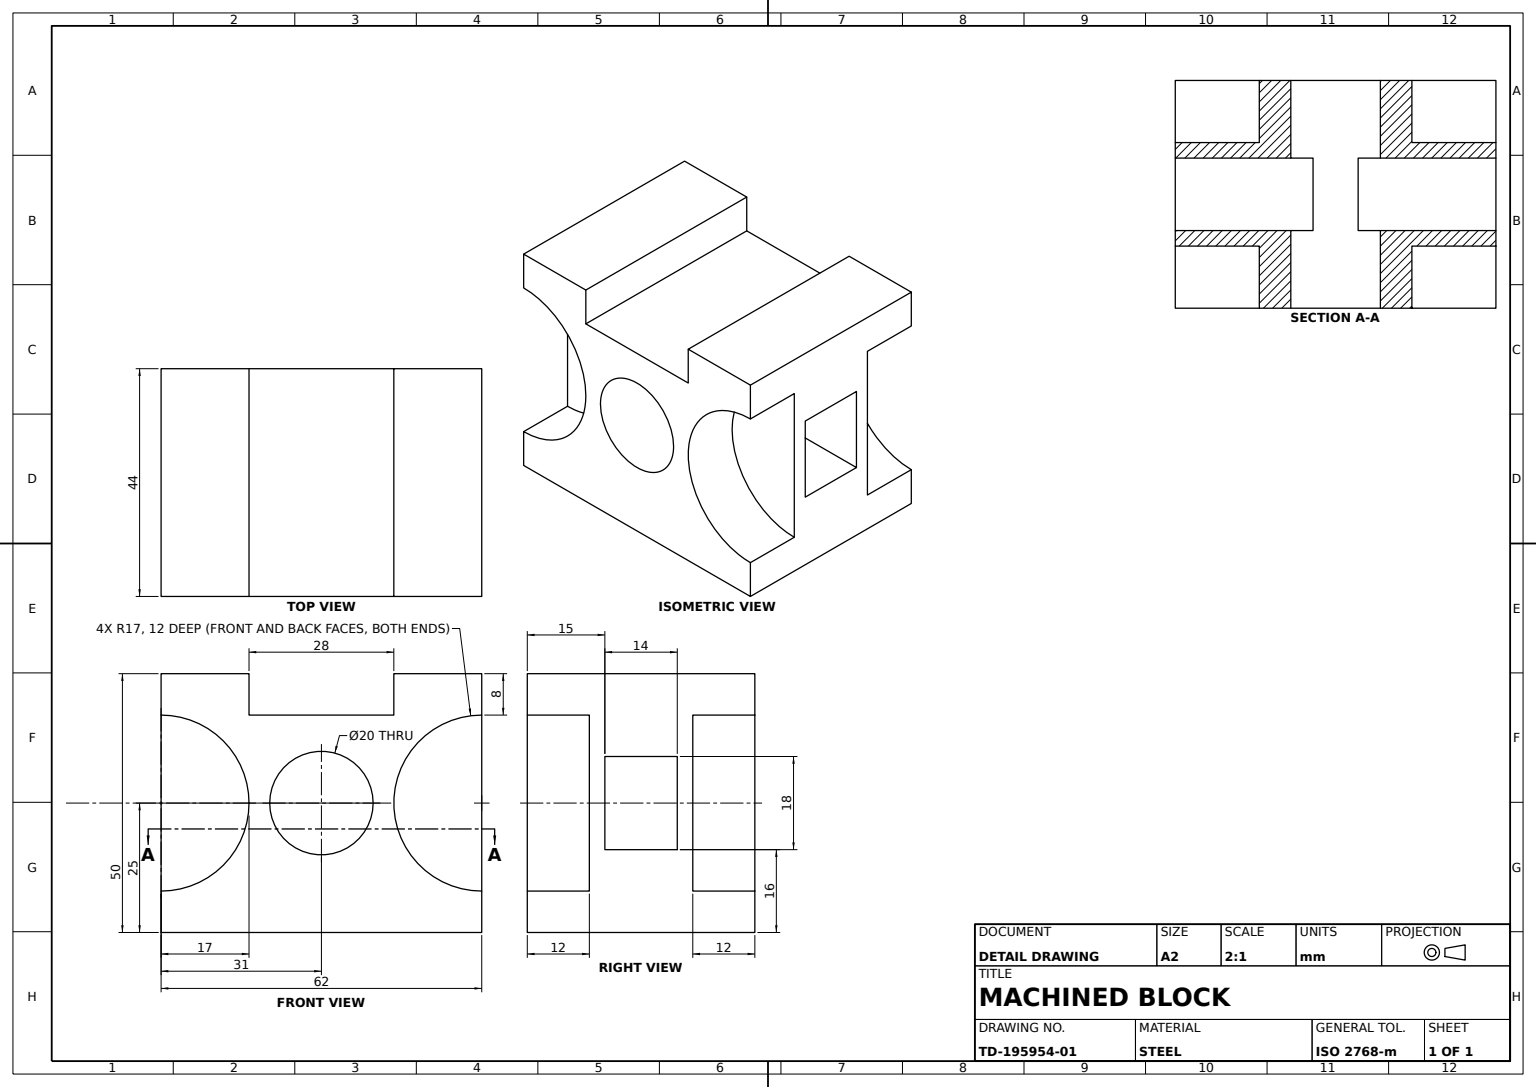
from build123d import *

# Parameters (mm, degrees)
BLOCK_PROFILE_SKETCH_W     = 62
BLOCK_PROFILE_SKETCH_H     = 50
BLOCK_62X50X44_DEPTH       = 44
THROUGH_HOLE_SKETCH_R      = 10
THROUGH_HOLE_20_DEPTH      = 44
TOP_SLOT_34X12_DEPTH       = 12
RELIEF_CUT_A_DEPTH         = 12
SIDE_RELIEF_CUT_DEPTH      = 60.3464405
SIDE_RELIEF_CUT_DEPTH_BACK = 60.3464405
RELIEF_START               = -12
RELIEF_CUT_B_DEPTH         = 12
RELIEF_CUT_C_DEPTH         = 12
WINDOW_SKETCH_W            = 14
WINDOW_SKETCH_H            = 18
WINDOW_CUT_DEPTH           = 81.031243899


with BuildPart() as part:
    # Block Profile Sketch → Block 62x50x44 (new body)
    with BuildSketch(Plane.XY):
        Rectangle(BLOCK_PROFILE_SKETCH_W, BLOCK_PROFILE_SKETCH_H)
    extrude(amount=BLOCK_62X50X44_DEPTH)

    # Through Hole Sketch → Through Hole Ø20 (cut)
    with BuildSketch(Plane.XY.offset(44)):
        Circle(THROUGH_HOLE_SKETCH_R)
    extrude(amount=-THROUGH_HOLE_20_DEPTH, mode=Mode.SUBTRACT)

    # Top Slot Sketch → Top Slot 34x12 (cut)
    with BuildSketch(Plane.XY.offset(44)):
        with BuildLine():
            Line((31, 17), (31, -17))
            ThreePointArc((31, -17), (14, 0), (31, 17))
        make_face()
    extrude(amount=-TOP_SLOT_34X12_DEPTH, mode=Mode.SUBTRACT)

    # Relief Cut A Sketch → Relief Cut A (cut)
    with BuildSketch(Plane.XY.offset(44)):
        with BuildLine():
            Line((31, -17), (31, 17))
            ThreePointArc((31, 17), (14, 0), (31, -17))
        make_face()
        with BuildLine():
            Line((-31, -17), (-31, 17))
            ThreePointArc((-31, 17), (-14, 0), (-31, -17))
        make_face()
    extrude(amount=-RELIEF_CUT_A_DEPTH, mode=Mode.SUBTRACT)

    # Side Relief Sketch → Side Relief Cut (cut, two sides: drawn at the far end of the back side and taken through both)
    with BuildSketch(Plane.XY.offset(44).offset(-SIDE_RELIEF_CUT_DEPTH_BACK)):
        Polygon((-14, 169.536240471), (-14, 25), (-14, 17), (14, 17), (14, 25), (14, 169.536240471), (14, 458.608721412), (-14, 458.608721412), align=None)
    extrude(amount=SIDE_RELIEF_CUT_DEPTH + SIDE_RELIEF_CUT_DEPTH_BACK, mode=Mode.SUBTRACT)

    # Relief Cut B Sketch → Relief Cut B (cut)
    with BuildSketch(Plane(origin=(0, 0, 0), x_dir=(-1, 0, 0), z_dir=(0, 0, -1)).offset(RELIEF_START)):
        with BuildLine():
            ThreePointArc((31, 17), (14, 0), (31, -17))
            Line((31, -17), (31, 17))
        make_face()
    extrude(amount=RELIEF_CUT_B_DEPTH, mode=Mode.SUBTRACT)

    # Relief Cut C Sketch → Relief Cut C (cut)
    with BuildSketch(Plane(origin=(0, 0, 0), x_dir=(-1, 0, 0), z_dir=(0, 0, -1)).offset(RELIEF_START)):
        with BuildLine():
            ThreePointArc((-31, -17), (-14, 0), (-31, 17))
            Line((-31, 17), (-31, -17))
        make_face()
    extrude(amount=RELIEF_CUT_C_DEPTH, mode=Mode.SUBTRACT)

    # Window Sketch → Window Cut (cut, through all)
    with BuildSketch(Plane.ZY.offset(31)):
        with Locations((22, 0)):
            Rectangle(WINDOW_SKETCH_W, WINDOW_SKETCH_H)
    extrude(amount=-WINDOW_CUT_DEPTH, mode=Mode.SUBTRACT)


solid = part.part
